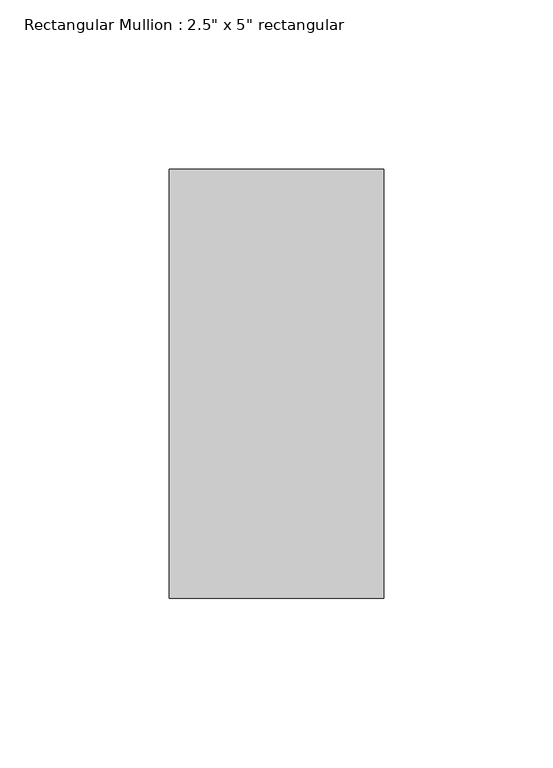
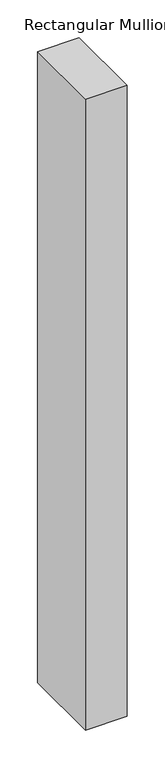
"""IFC4 building model written with IfcOpenShell, lengths in millimetres: member geometry."""

from ifc_helpers import new_model, si_unit, frame, origin, place, context, project, spatial, polyline, outline, extrude, source, transform, mapped, element, save


def member_870cb0cc(model_context):
    return source(origin(), model_context, "Body", "SweptSolid", [
        extrude(outline(polyline([(0.0, 63.5), (0.0, -63.5), (-63.5, -63.5), (-63.5, 63.5), (0.0, 63.5)])), frame((0.0, 0.0, -1019.953622), z_axis=(0.0, 0.0, 1.0), x_axis=(1.0, 0.0, 0.0)), (0.0, 0.0, 1.0), 1019.953622),
    ])


if __name__ == "__main__":
    model = new_model("IFC4")
    model_context = context("Model", 3, world=origin())
    ifc_project = project(units=[si_unit("LENGTHUNIT", "METRE", prefix="MILLI")], contexts=[model_context])
    site = spatial("IfcSite", under=ifc_project)
    building = spatial("IfcBuilding", under=site)
    placement = place(None, origin())
    member_shape = member_870cb0cc(model_context)
    element("IfcMember", 1, ObjectType="Rectangular Mullion : 2.5\" x 5\" rectangular", at=placement, inside=building, context=model_context, shape_type="MappedRepresentation", body=[
        mapped(member_shape, transform((0.0, 0.0, 0.0), x_axis=(1.0, 0.0, 0.0), y_axis=(0.0, 1.0, 0.0), z_axis=(0.0, 0.0, 1.0))),
    ])
    save(model, "model.ifc")

# Revit data of these elements
# Type "Rectangular Mullion : 2.5\" x 5\" rectangular"
#   built-in parameter 1007304 = 0.416667 (stored number, unit not read)
#   built-in parameter 1007301 = 0.104167 (stored number, unit not read)
#   built-in parameter 1007300 = 0.104167 (stored number, unit not read)
# Element 1 (IfcMember, "Rectangular Mullion : 2.5\" x 5\" rectangular")
#   Materials on its faces: "Aluminum"
# Materials
#   "Aluminum": class "Metal", colour RGB 247 247 247, transparency 0, Description = "Aluminum 6061", Cost = 0
